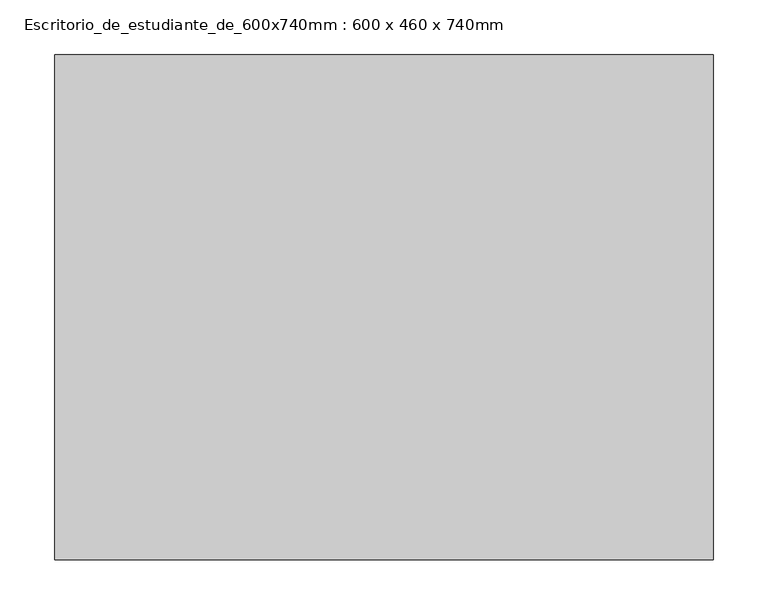
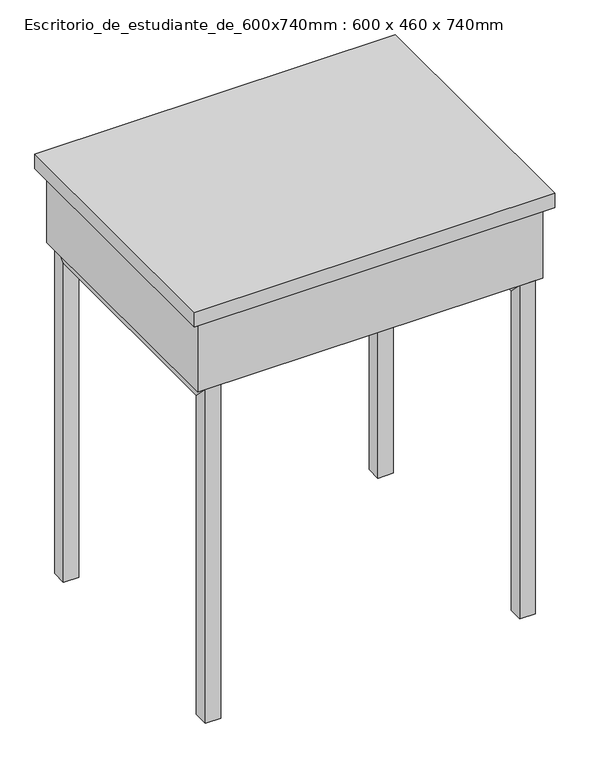
"""IFC4 building model written with IfcOpenShell, lengths in millimetres: furniture geometry, Escritorio_de_estudiante_de_600x740mm : 600 x 460 x 740mm."""

from ifc_helpers import new_model, si_unit, frame, origin, place, context, project, spatial, polyline, outline, extrude, faceted_brep, source, transform, mapped, element, save


def escritorio_de_estudiante_de_600x740mm_600_x_460_x_740mm_3f482482(model_context):
    return source(origin(), model_context, "Body", "SolidModel", [
        extrude(outline(polyline([(300.0, 230.0), (300.0, -230.0), (-300.0, -230.0), (-300.0, 230.0), (300.0, 230.0)])), frame((0.0, 0.0, 714.6), z_axis=(0.0, 0.0, 1.0), x_axis=(1.0, 0.0, 0.0)), (0.0, 0.0, 1.0), 25.4),
        extrude(outline(polyline([(287.3, 217.3), (287.3, -217.3), (-287.3, -217.3), (-287.3, 217.3), (287.3, 217.3)])), frame((0.0, 0.0, 587.6), z_axis=(0.0, 0.0, 1.0), x_axis=(1.0, 0.0, 0.0)), (0.0, 0.0, 1.0), 127.0),
        faceted_brep([(249.2, -217.3, 0.0), (249.2, -191.9, 0.0), (274.6, -191.9, 0.0), (274.6, -217.3, 0.0), (249.2, -217.3, 587.6), (249.2, -191.9, 562.2), (274.6, -191.9, 562.2), (274.6, -217.3, 587.6), (249.2, 217.3, 587.6), (249.2, 191.9, 562.2), (274.6, 191.9, 562.2), (274.6, 217.3, 587.6), (249.2, 217.3, 0.0), (274.6, 217.3, 0.0), (274.6, 191.9, 0.0), (249.2, 191.9, 0.0)], [[[0, 1, 2, 3]], [[1, 0, 4, 5]], [[2, 1, 5, 6]], [[3, 2, 6, 7]], [[0, 3, 7, 4]], [[5, 4, 8, 9]], [[6, 5, 9, 10]], [[7, 6, 10, 11]], [[4, 7, 11, 8]], [[12, 13, 14, 15]], [[9, 8, 12, 15]], [[10, 9, 15, 14]], [[11, 10, 14, 13]], [[8, 11, 13, 12]]]),
        faceted_brep([(-249.2, -217.3, 0.0), (-274.6, -217.3, 0.0), (-274.6, -191.9, 0.0), (-249.2, -191.9, 0.0), (-249.2, -217.3, 587.6), (-274.6, -217.3, 587.6), (-274.6, -191.9, 562.2), (-249.2, -191.9, 562.2), (-249.2, 217.3, 587.6), (-274.6, 217.3, 587.6), (-274.6, 191.9, 562.2), (-249.2, 191.9, 562.2), (-249.2, 217.3, 0.0), (-249.2, 191.9, 0.0), (-274.6, 191.9, 0.0), (-274.6, 217.3, 0.0)], [[[0, 1, 2, 3]], [[1, 0, 4, 5]], [[2, 1, 5, 6]], [[3, 2, 6, 7]], [[0, 3, 7, 4]], [[5, 4, 8, 9]], [[6, 5, 9, 10]], [[7, 6, 10, 11]], [[4, 7, 11, 8]], [[12, 13, 14, 15]], [[9, 8, 12, 15]], [[10, 9, 15, 14]], [[11, 10, 14, 13]], [[8, 11, 13, 12]]]),
    ])


if __name__ == "__main__":
    model = new_model("IFC4")
    model_context = context("Model", 3, world=origin())
    ifc_project = project(units=[si_unit("LENGTHUNIT", "METRE", prefix="MILLI")], contexts=[model_context])
    site = spatial("IfcSite", under=ifc_project)
    building = spatial("IfcBuilding", under=site)
    placement = place(None, origin())
    escritorio_de_estudiante_de_600x740mm_600_x_460_x_740mm_shape = escritorio_de_estudiante_de_600x740mm_600_x_460_x_740mm_3f482482(model_context)
    element("IfcFurniture", 1, ObjectType="Escritorio_de_estudiante_de_600x740mm : 600 x 460 x 740mm", at=placement, inside=building, context=model_context, shape_type="MappedRepresentation", body=[
        mapped(escritorio_de_estudiante_de_600x740mm_600_x_460_x_740mm_shape, transform((0.0, 0.0, 0.0), x_axis=(1.0, 0.0, 0.0), y_axis=(0.0, 1.0, 0.0), z_axis=(0.0, 0.0, 1.0))),
    ])
    save(model, "model.ifc")

# Revit data of these elements
# Type "Escritorio_de_estudiante_de_600x740mm : 600 x 460 x 740mm"
#   ID_Source = "BIMTOOL"
#   ID_Objeto = "BT_F_G_836"
#   BT_Web_del_Producto = "http://www.bimtool.com/Catalog.aspx?categoria=ESCRITORIOS"
#   BT_Uso = "Interior"
#   BT_SKU = "00 00 00"
#   BT_Profundidad = "460mm"
#   BT_Peso = "N/a"
#   BT_Nombre_Técnico = "Escritorio de estudiante de 600x740mm"
#   BT_Nombre_Corto = "Escritorio de estudiante de 600x740mm"
#   BT_Material = "Madera - Acero"
#   BT_MasterFormat® = "12 00 00"
#   BT_Marca = "Bimtool"
#   BT_Itemizado_Estandar_CDT = "H 06 06 00"
#   BT_Fabricante = "Bimtool"
#   BT_Especialidad = "Mobiliario e Interiorismo"
#   BT_Elemento = "Escritorios"
#   BT_EETT = "Escritorio de estudiante de 600x740mm, con 4 apoyos de acero"
#   BT_Descripción = "Escritorio de madera"
#   BT_Código_Origen = ""
#   BT_Código_Línea = "Línea"
#   BT_Color = "N/a"
#   BT_Ancho = "600mm"
#   BT_Alto = "740mm"
#   Depth = 460 mm
#   Height = 740 mm
#   Width = 600 mm
#   Default Elevation = 0
#   Assembly Code = ""
# Element 1 (IfcFurniture, "Escritorio_de_estudiante_de_600x740mm : 600 x 460 x 740mm")
#   Materials on its faces: "Metal - Chrome", "Wood - Birch", "Metal - Steel"
# Materials
#   "Metal - Chrome": colour RGB 201 201 201, transparency 0
#   "Wood - Birch": colour RGB 210 159 95, transparency 0
#   "Metal - Steel": colour RGB 247 247 247, transparency 0
